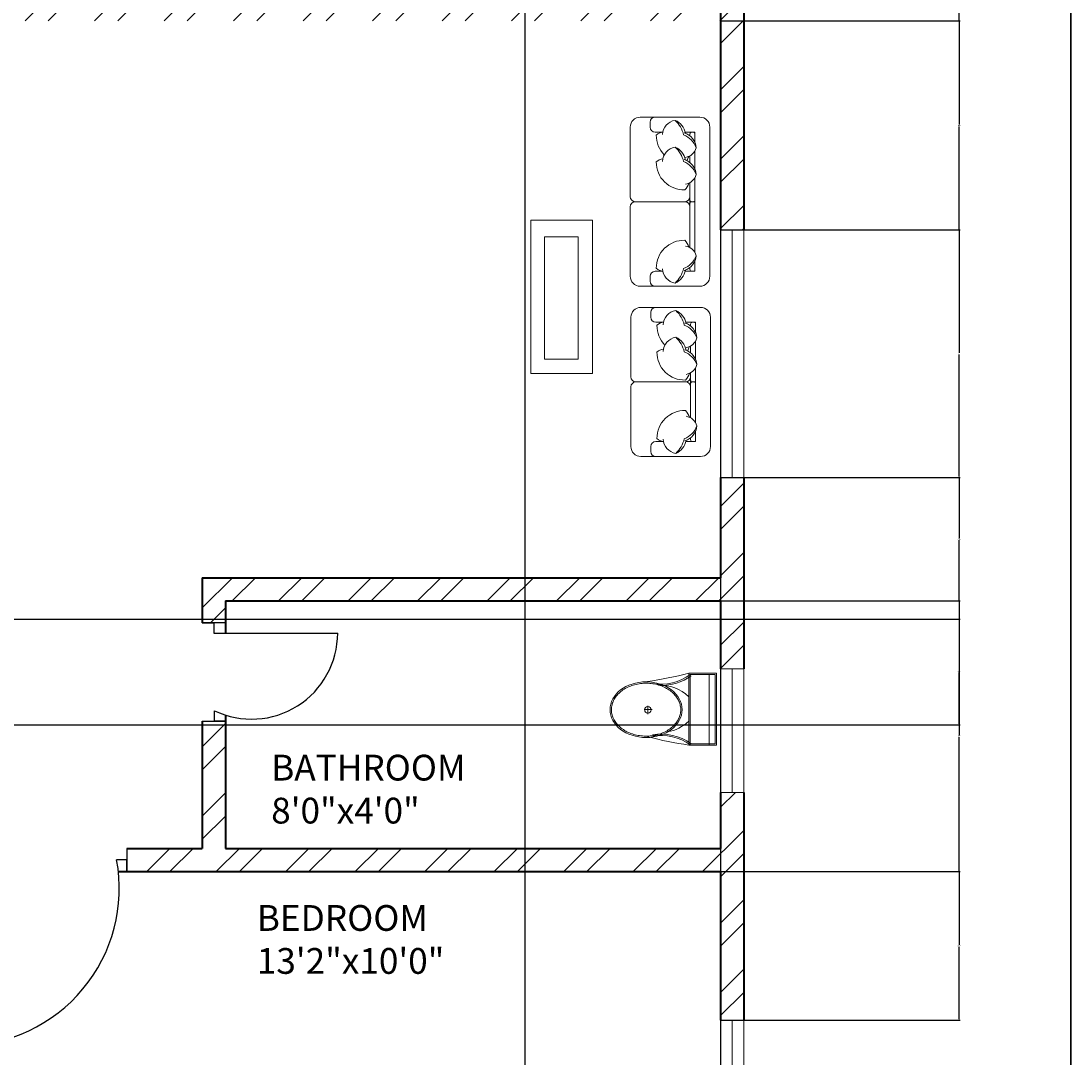
# Model space of a CAD drawing. Units: inches. Extents: x 2063 to 2617, y 1299 to 2210.
# Tile 5 of 22: x 2414 to 2617, y 1526 to 1727. Entities that reach past the tile are written whole.
import ezdxf

# ---------------------------------------------------------------- set-up
doc = ezdxf.new("R2010")
doc.units = ezdxf.units.IN
for name, color, linetype, lineweight in [('A-ANNO-DIMS', 2, 'Continuous', 18), ('A-ANNO-TTLB', 7, 'Continuous', 35), ('A-AREA-IDEN', 7, 'Continuous', 18), ('A-DOOR', 11, 'Continuous', 25), ('A-FLOR-FIXT', 8, 'Continuous', 18), ('A-FURN', 8, 'Continuous', 18), ('A-GLAZ', 123, 'Continuous', 18), ('A-WALL', 7, 'Continuous', 40)]:
    doc.layers.add(name, color=color, linetype=linetype, lineweight=lineweight)
doc.layers.add('A-WALL-PATT', color=215, linetype='Continuous', lineweight=13, true_color=0xa953a0)
doc.styles.get("Standard").update_dxf_attribs({"font": 'arial.ttf'})
doc.dimstyles.get("Standard").update_dxf_attribs({"dimtxt": 0.18, "dimasz": 0.18, "dimexe": 0.18, "dimexo": 0.0625, "dimgap": 0.09, "dimtad": 0, "dimtih": 1, "dimtoh": 1, "dimdec": 4, "dimzin": 0, "dimdsep": 46, "dimtxsty": 'Standard', "dimcen": 0.09, "dimadec": 0, "dimazin": 0, "dimtfac": 1, "dimtdec": 4, "dimtofl": 0, "dimtmove": 0, "dimatfit": 3, "dimfxl": 1, "dimtolj": 1, "dimtzin": 0, "dimarcsym": 0})

# ---------------------------------------------------------------- blocks, each defined once
blk = doc.blocks.new('A$C31115884')
for p, q in [((283.1, 497.7), (223.4, 497.7)), ((257.5, 466.4), (257.5, 523.2)), ((0, 200), (0, 0)), ((520, 200), (0, 200)), ((10, 190), (10, 10)), ((510, 190), (10, 190)), ((510, 10), (510, 190)), ((520, 0), (520, 200)), ((510, 54.5), (0, 54.5)), ((10, 10), (510, 10)), ((0, 0), (520, 0))]:
    blk.add_line(p, q)
blk.add_circle((255.6, 496.4), 23.6)
for centre, radius, start, end in [((2777.7, -204.6), 2807, 165.4549, 171.71327), ((-294.5, 403.3), 364.7, 324.20913, 9.34987), ((-294.5, 403.3), 374.7, 324.20913, 9.34987), ((805.8, 403.3), 364.7, 170.65013, 215.79087), ((3237, 905), 2807, 188.28673, 194.5451), ((139.5, 406.2), 293.5, 315.84364, 2.65635), ((805.8, 403.3), 374.7, 179.20365, 215.79087), ((383.6, 406.2), 293.5, 190.27735, 224.15636)]:
    blk.add_arc(centre, radius, start, end)
blk.add_ellipse((256.2, 509.9), major_axis=(0, -260.7), ratio=0.772727)
blk.add_open_spline([(256.2, 259.2), (263.1, 259.2), (270, 259.7), (287.8, 262.3), (298.7, 265.1), (319.9, 273.1), (330.2, 278.4), (350.1, 291.1), (359.7, 298.7), (377.7, 315.9), (386.2, 325.5), (401.7, 346.6), (408.8, 358.1), (421.3, 382.5), (426.8, 395.5), (435.9, 422.4), (439.5, 436.4), (444.8, 465.1), (446.5, 479.7), (447.9, 509.2), (447.6, 524), (445, 553.3), (442.7, 567.8), (436.3, 596), (432.1, 609.7), (421.9, 636), (416, 648.6), (402.5, 672.1), (395, 683), (378.6, 703), (369.8, 712.1), (351.1, 728), (341.3, 734.8), (320.9, 746.2), (310.4, 750.7), (288.9, 757.3), (278, 759.4), (256, 761), (245, 760.6), (223.1, 757.2), (212.3, 754.3), (191.1, 746.1), (180.8, 740.7), (160.9, 727.8), (151.4, 720.1), (133.5, 702.7), (125.1, 693), (109.6, 671.7), (102.6, 660.2), (90.2, 635.7), (84.9, 622.7), (76, 595.6), (72.4, 581.6), (67.2, 552.9), (65.6, 538.2), (64.4, 508.8), (64.8, 494), (67.5, 464.7), (69.9, 450.2), (76.6, 422), (80.8, 408.3), (91.1, 382.2), (97.2, 369.7), (110.8, 346.3), (118.4, 335.4), (134.8, 315.6), (143.7, 306.7), (162.4, 290.9), (172.3, 284.2), (192.8, 273), (203.3, 268.6), (224.8, 262.2), (235.8, 260.2), (249.9, 259.3), (253, 259.2), (256.2, 259.2)], degree=3, knots=[0, 0, 0, 0, 0.110105, 0.110105, 0.285049, 0.285049, 0.459994, 0.459994, 0.634938, 0.634938, 0.809882, 0.809882, 0.984827, 0.984827, 1.159771, 1.159771, 1.334715, 1.334715, 1.50966, 1.50966, 1.684604, 1.684604, 1.859549, 1.859549, 2.034493, 2.034493, 2.209437, 2.209437, 2.384382, 2.384382, 2.559326, 2.559326, 2.73427, 2.73427, 2.909215, 2.909215, 3.084159, 3.084159, 3.259103, 3.259103, 3.434048, 3.434048, 3.608992, 3.608992, 3.783936, 3.783936, 3.958881, 3.958881, 4.133825, 4.133825, 4.30877, 4.30877, 4.483714, 4.483714, 4.658658, 4.658658, 4.833603, 4.833603, 5.008547, 5.008547, 5.183491, 5.183491, 5.358436, 5.358436, 5.53338, 5.53338, 5.708324, 5.708324, 5.883269, 5.883269, 6.058213, 6.058213, 6.233158, 6.233158, 6.283185, 6.283185, 6.283185, 6.283185])
blk = doc.blocks.new('WIN-24IN')
for p, q in [((0, 24), (4.5, 24)), ((0, 24), (0, 0)), ((4.5, 24), (2.25, 24)), ((2.25, 24), (2.25, 0)), ((4.5, 24), (4.5, 0)), ((2.25, 0), (0, 0)), ((0, 0), (4.5, 0))]:
    blk.add_line(p, q)
blk = doc.blocks.new('TABLE-COFFEE')
for points in [[(0, 29.74), (11.98, 29.74), (11.98, 0), (0, 0)], [(2.66, 26.46), (2.66, 26.46), (2.66, 26.46), (2.66, 26.46)], [(2.66, 26.46), (2.66, 26.46), (2.66, 26.46), (2.66, 26.46)], [(2.66, 26.46), (2.66, 26.46), (2.66, 26.46), (2.66, 26.46)], [(2.66, 26.46), (9.18, 26.46), (9.18, 2.77), (2.66, 2.77)]]:
    blk.add_lwpolyline(points, close=True)
blk = doc.blocks.new('*D38')
at = {"layer": 'A-ANNO-DIMS', "color": 0, "lineweight": -2, "transparency": 16777216}
for p, q in [((2549.21, 1562.31), (2595.57, 1562.31)), ((2595.39, 1562.13), (2595.39, 1548.08)), ((2595.39, 1533.66), (2595.39, 1547.71)), ((2549.21, 1533.48), (2595.57, 1533.48))]:
    blk.add_line(p, q, dxfattribs=at)
at = {"layer": 'A-ANNO-DIMS', "color": 0, "transparency": 16777216}
for points in [[(2595.36, 1562.13), (2595.42, 1562.13), (2595.39, 1562.31)], [(2595.36, 1533.66), (2595.42, 1533.66), (2595.39, 1533.48)]]:
    blk.add_solid(points, dxfattribs=at)
at = {"layer": 'Defpoints', "color": 0, "transparency": 16777216}
for p in [(2549.14, 1562.31), (2595.39, 1562.31), (2549.14, 1533.48)]:
    blk.add_point(p, dxfattribs=at)
at = {"layer": 'A-ANNO-DIMS', "color": 0, "transparency": 16777216, "insert": (2595.39, 1547.9), "char_height": 0.18, "attachment_point": 5}
blk.add_mtext('\\A1;28.83', dxfattribs=at)
blk = doc.blocks.new('*D39')
at = {"layer": 'A-ANNO-DIMS', "color": 0, "lineweight": -2, "transparency": 16777216}
for p, q in [((2549.21, 1614.81), (2595.57, 1614.81)), ((2595.39, 1614.63), (2595.39, 1588.74)), ((2595.39, 1562.49), (2595.39, 1588.38)), ((2549.21, 1562.31), (2595.57, 1562.31))]:
    blk.add_line(p, q, dxfattribs=at)
at = {"layer": 'A-ANNO-DIMS', "color": 0, "transparency": 16777216}
for points in [[(2595.36, 1614.63), (2595.42, 1614.63), (2595.39, 1614.81)], [(2595.36, 1562.49), (2595.42, 1562.49), (2595.39, 1562.31)]]:
    blk.add_solid(points, dxfattribs=at)
at = {"layer": 'Defpoints', "color": 0, "transparency": 16777216}
for p in [(2549.14, 1614.81), (2595.39, 1614.81), (2549.14, 1562.31)]:
    blk.add_point(p, dxfattribs=at)
at = {"layer": 'A-ANNO-DIMS', "color": 0, "transparency": 16777216, "insert": (2595.39, 1588.56), "char_height": 0.18, "attachment_point": 5}
blk.add_mtext('\\A1;52.5', dxfattribs=at)
blk = doc.blocks.new('*D40')
at = {"layer": 'A-ANNO-DIMS', "color": 0, "lineweight": -2, "transparency": 16777216}
for p, q in [((2549.21, 1638.78), (2595.57, 1638.78)), ((2595.39, 1638.6), (2595.39, 1626.98)), ((2595.39, 1614.99), (2595.39, 1626.61)), ((2549.21, 1614.81), (2595.57, 1614.81))]:
    blk.add_line(p, q, dxfattribs=at)
at = {"layer": 'A-ANNO-DIMS', "color": 0, "transparency": 16777216}
for points in [[(2595.36, 1638.6), (2595.42, 1638.6), (2595.39, 1638.78)], [(2595.36, 1614.99), (2595.42, 1614.99), (2595.39, 1614.81)]]:
    blk.add_solid(points, dxfattribs=at)
at = {"layer": 'Defpoints', "color": 0, "transparency": 16777216}
for p in [(2549.14, 1638.78), (2595.39, 1638.78), (2549.14, 1614.81)]:
    blk.add_point(p, dxfattribs=at)
at = {"layer": 'A-ANNO-DIMS', "color": 0, "transparency": 16777216, "insert": (2595.39, 1626.79), "char_height": 0.18, "attachment_point": 5}
blk.add_mtext('\\A1;23.965', dxfattribs=at)
blk = doc.blocks.new('*D41')
at = {"layer": 'A-ANNO-DIMS', "color": 0, "lineweight": -2, "transparency": 16777216}
for p, q in [((2549.21, 1686.78), (2595.57, 1686.78)), ((2595.39, 1686.6), (2595.39, 1662.96)), ((2595.39, 1638.96), (2595.39, 1662.59)), ((2549.21, 1638.78), (2595.57, 1638.78))]:
    blk.add_line(p, q, dxfattribs=at)
at = {"layer": 'A-ANNO-DIMS', "color": 0, "transparency": 16777216}
for points in [[(2595.36, 1686.6), (2595.42, 1686.6), (2595.39, 1686.78)], [(2595.36, 1638.96), (2595.42, 1638.96), (2595.39, 1638.78)]]:
    blk.add_solid(points, dxfattribs=at)
at = {"layer": 'Defpoints', "color": 0, "transparency": 16777216}
for p in [(2549.14, 1686.78), (2595.39, 1686.78), (2549.14, 1638.78)]:
    blk.add_point(p, dxfattribs=at)
at = {"layer": 'A-ANNO-DIMS', "color": 0, "transparency": 16777216, "insert": (2595.39, 1662.78), "char_height": 0.18, "attachment_point": 5}
blk.add_mtext('\\A1;48', dxfattribs=at)
blk = doc.blocks.new('*D42')
at = {"layer": 'A-ANNO-DIMS', "color": 0, "lineweight": -2, "transparency": 16777216}
for p, q in [((2549.21, 1727.31), (2595.57, 1727.31)), ((2595.39, 1727.13), (2595.39, 1707.23)), ((2595.39, 1686.96), (2595.39, 1706.86)), ((2549.21, 1686.78), (2595.57, 1686.78))]:
    blk.add_line(p, q, dxfattribs=at)
at = {"layer": 'A-ANNO-DIMS', "color": 0, "transparency": 16777216}
for points in [[(2595.36, 1727.13), (2595.42, 1727.13), (2595.39, 1727.31)], [(2595.36, 1686.96), (2595.42, 1686.96), (2595.39, 1686.78)]]:
    blk.add_solid(points, dxfattribs=at)
at = {"layer": 'Defpoints', "color": 0, "transparency": 16777216}
for p in [(2549.14, 1727.31), (2595.39, 1727.31), (2549.14, 1686.78)]:
    blk.add_point(p, dxfattribs=at)
at = {"layer": 'A-ANNO-DIMS', "color": 0, "transparency": 16777216, "insert": (2595.39, 1707.04), "char_height": 0.18, "attachment_point": 5}
blk.add_mtext('\\A1;40.535', dxfattribs=at)
blk = doc.blocks.new('*D43')
at = {"layer": 'A-ANNO-DIMS', "color": 0, "lineweight": -2, "transparency": 16777216}
for p, q in [((2549.21, 1766.03), (2595.57, 1766.03)), ((2595.39, 1765.85), (2595.39, 1746.85)), ((2595.39, 1727.49), (2595.39, 1746.49)), ((2549.21, 1727.31), (2595.57, 1727.31))]:
    blk.add_line(p, q, dxfattribs=at)
at = {"layer": 'A-ANNO-DIMS', "color": 0, "transparency": 16777216}
for points in [[(2595.36, 1765.85), (2595.42, 1765.85), (2595.39, 1766.03)], [(2595.36, 1727.49), (2595.42, 1727.49), (2595.39, 1727.31)]]:
    blk.add_solid(points, dxfattribs=at)
at = {"layer": 'Defpoints', "color": 0, "transparency": 16777216}
for p in [(2549.14, 1766.03), (2595.39, 1766.03), (2549.14, 1727.31)]:
    blk.add_point(p, dxfattribs=at)
at = {"layer": 'A-ANNO-DIMS', "color": 0, "transparency": 16777216, "insert": (2595.39, 1746.67), "char_height": 0.18, "attachment_point": 5}
blk.add_mtext('\\A1;38.72', dxfattribs=at)
blk = doc.blocks.new('*D52')
at = {"layer": 'A-ANNO-DIMS', "color": 0, "lineweight": -2, "transparency": 16777216}
for p, q in [((2511.17, 2124.25), (2511.17, 1317.7)), ((2549.14, 2124.25), (2549.14, 1317.7)), ((2511.35, 1317.88), (2529.69, 1317.88)), ((2548.96, 1317.88), (2530.62, 1317.88))]:
    blk.add_line(p, q, dxfattribs=at)
at = {"layer": 'A-ANNO-DIMS', "color": 0, "transparency": 16777216}
for points in [[(2511.35, 1317.91), (2511.35, 1317.85), (2511.17, 1317.88)], [(2548.96, 1317.91), (2548.96, 1317.85), (2549.14, 1317.88)]]:
    blk.add_solid(points, dxfattribs=at)
at = {"layer": 'Defpoints', "color": 0, "transparency": 16777216}
for p in [(2511.17, 2124.31), (2549.14, 2124.31), (2549.14, 1317.88)]:
    blk.add_point(p, dxfattribs=at)
at = {"layer": 'A-ANNO-DIMS', "color": 0, "transparency": 16777216, "insert": (2530.16, 1317.88), "char_height": 0.18, "attachment_point": 5}
blk.add_mtext('\\A1;37.974', dxfattribs=at)
blk = doc.blocks.new('*D68')
at = {"layer": 'A-ANNO-DIMS', "color": 0, "lineweight": -2, "transparency": 16777216}
for p, q in [((2228.21, 1611.27), (2595.57, 1611.27)), ((2595.39, 1611.09), (2595.39, 1601.22)), ((2595.39, 1590.99), (2595.39, 1600.86)), ((2228.21, 1590.81), (2595.57, 1590.81))]:
    blk.add_line(p, q, dxfattribs=at)
at = {"layer": 'A-ANNO-DIMS', "color": 0, "transparency": 16777216}
for points in [[(2595.36, 1611.09), (2595.42, 1611.09), (2595.39, 1611.27)], [(2595.36, 1590.99), (2595.42, 1590.99), (2595.39, 1590.81)]]:
    blk.add_solid(points, dxfattribs=at)
at = {"layer": 'Defpoints', "color": 0, "transparency": 16777216}
for p in [(2228.14, 1611.27), (2595.39, 1611.27), (2228.14, 1590.81)]:
    blk.add_point(p, dxfattribs=at)
at = {"layer": 'A-ANNO-DIMS', "color": 0, "transparency": 16777216, "insert": (2595.39, 1601.04), "char_height": 0.18, "attachment_point": 5}
blk.add_mtext('\\A1;20.46', dxfattribs=at)

msp = doc.modelspace()

# ---------------------------------------------------------------- hatches: boundary and pattern name
at = {"layer": 'A-WALL-PATT'}
h = msp.add_hatch(dxfattribs=at)
h.set_pattern_fill('ANSI32', color=256)
h.paths.add_polyline_path([(2553.6442, 2128.8122), (2511.1703, 2128.8122), (2511.1703, 2124.3122), (2549.1442, 2124.3122), (2549.1442, 2095.662), (2553.6442, 2095.662)])
h.paths.add_polyline_path([(2553.6442, 2035.662), (2549.1442, 2035.662), (2549.1442, 1980.3122), (2503.7214, 1980.3122), (2503.7214, 1975.8122), (2549.1442, 1975.8122), (2549.1442, 1962.9693), (2553.6442, 1962.9693)])
h.paths.add_polyline_path([(2553.6442, 1938.9693), (2549.1442, 1938.9693), (2549.1442, 1927.8122), (2477.1442, 1927.8122), (2477.1442, 1975.8122), (2481.2918, 1975.8122), (2481.2918, 1980.3122), (2453.2648, 1980.3122), (2453.2648, 1975.8122), (2472.6442, 1975.8122), (2472.6442, 1868.3122), (2400.6442, 1868.3122), (2400.6442, 1861.3782), (2405.1442, 1861.3782), (2405.1442, 1863.8122), (2480.9699, 1863.8122), (2480.9699, 1866.0622), (2480.9699, 1868.3122), (2477.1442, 1868.3122), (2477.1442, 1923.3122), (2549.1442, 1923.3122), (2549.1442, 1908.8504), (2553.6442, 1908.8504)])
h.paths.add_polyline_path([(2553.6442, 1884.8504), (2549.1442, 1884.8504), (2549.1442, 1868.3122), (2501.0636, 1868.3122), (2501.0636, 1863.8122), (2549.1442, 1863.8122), (2549.1442, 1826.0298), (2553.6442, 1826.0298)])
h.paths.add_polyline_path([(2388.1504, 1980.3122), (2340.6442, 1980.3122), (2340.6442, 2124.3122), (2358.7501, 2124.3122), (2358.7501, 2128.8122), (2316.3482, 2128.8122), (2316.3482, 2124.3122), (2336.1442, 2124.3122), (2336.1442, 1980.3122), (2289.1737, 1980.3122), (2289.1737, 1975.8122), (2336.1442, 1975.8122), (2336.1442, 1619.3122), (2333.1433, 1619.3122), (2333.1433, 1614.8122), (2344.1671, 1614.8122), (2344.1671, 1617.0622), (2344.1671, 1619.3122), (2340.6442, 1619.3122), (2340.6442, 1975.8122), (2388.1504, 1975.8122), (2388.1504, 1978.0622)])
h.paths.add_polyline_path([(2290.1442, 1614.8122), (2301.4594, 1614.8122), (2301.4594, 1617.0622), (2301.4594, 1619.3122), (2285.6442, 1619.3122), (2285.6442, 1566.8122), (2280.8619, 1566.8122), (2280.8619, 1564.5622), (2280.8619, 1562.3122), (2285.6442, 1562.3122), (2285.6442, 1442.3122), (2281.7879, 1442.3122), (2281.7879, 1437.8122), (2285.6442, 1437.8122), (2285.6442, 1401.8122), (2290.1442, 1401.8122)])
h.paths.add_polyline_path([(2549.1442, 1731.8122), (2405.1442, 1731.8122), (2405.1442, 1834.4638), (2402.8942, 1834.4638), (2400.6442, 1834.4638), (2400.6442, 1727.3122), (2549.1442, 1727.3122)])
h.paths.add_polyline_path([(2553.6442, 1766.0298), (2551.3942, 1766.0298), (2549.1442, 1766.0298), (2549.1442, 1686.7767), (2553.6442, 1686.7767)])
h.paths.add_polyline_path([(2553.6442, 1638.7767), (2551.3942, 1638.7767), (2549.1442, 1638.7767), (2549.1442, 1619.3122), (2448.6442, 1619.3122), (2448.6442, 1610.5671), (2450.8942, 1610.5671), (2453.1442, 1610.5671), (2453.1442, 1614.8122), (2549.1442, 1614.8122), (2549.1442, 1601.6421), (2553.6442, 1601.6421)])
h.paths.add_polyline_path([(2553.6442, 1577.6421), (2551.3942, 1577.6421), (2549.1442, 1577.6421), (2549.1442, 1566.8122), (2453.1442, 1566.8122), (2453.1442, 1591.5045), (2451.0335, 1591.5045), (2448.6442, 1591.5045), (2448.6442, 1566.8122), (2434.0475, 1566.8122), (2434.0475, 1562.3122), (2549.1442, 1562.3122), (2549.1442, 1533.48), (2553.6442, 1533.48)])
h.paths.add_polyline_path([(2553.6442, 1473.48), (2549.1442, 1473.48), (2549.1442, 1442.3122), (2502.6258, 1442.3122), (2502.6258, 1437.8122), (2549.1442, 1437.8122), (2549.1442, 1401.8122), (2553.6442, 1401.8122)])
h.paths.add_polyline_path([(2395.6442, 1562.3122), (2400.0901, 1562.3122), (2400.0901, 1564.5622), (2400.0901, 1566.8122), (2395.6442, 1566.8122), (2395.6442, 1619.3122), (2379.1127, 1619.3122), (2379.1127, 1614.8122), (2391.1442, 1614.8122), (2391.1442, 1401.8122), (2395.6442, 1401.8122), (2395.6442, 1437.8122), (2399.2425, 1437.8122), (2399.2425, 1440.0622), (2399.2425, 1442.3122), (2395.6442, 1442.3122)])
h.paths.add_polyline_path([(2442.6258, 1442.3122), (2419.6262, 1442.3122), (2419.6262, 1437.8122), (2442.6258, 1437.8122), (2442.6258, 1440.0622)])
h.paths.add_polyline_path([(2127.6442, 1480.2532), (2125.3942, 1480.2532), (2123.1442, 1480.2532), (2123.1442, 1401.8122), (2127.6442, 1401.8122), (2127.6442, 1437.8122), (2145.1538, 1437.8122), (2145.1538, 1440.0622), (2145.1538, 1442.3122), (2127.6442, 1442.3122)])
h.paths.add_polyline_path([(2259.809, 1442.3122), (2205.1538, 1442.3122), (2205.1538, 1437.8122), (2259.809, 1437.8122), (2259.809, 1440.0622)])
h.paths.add_polyline_path([(2127.6442, 1659.7652), (2123.1442, 1659.7652), (2123.1442, 1605.5161), (2125.3942, 1605.5161), (2127.6442, 1605.5161), (2127.6442, 1614.8122), (2223.6442, 1614.8122), (2223.6442, 1611.2723), (2228.1442, 1611.2723), (2228.1442, 1619.3122), (2127.6442, 1619.3122)])
h.paths.add_polyline_path([(2244.8673, 1566.8122), (2228.1442, 1566.8122), (2228.1442, 1590.8122), (2225.8942, 1590.8122), (2223.6442, 1590.8122), (2223.6442, 1566.8122), (2127.6442, 1566.8122), (2127.6442, 1581.5161), (2123.1442, 1581.5161), (2123.1442, 1540.2532), (2127.6442, 1540.2532), (2127.6442, 1562.3122), (2244.8673, 1562.3122), (2244.8673, 1564.5622)])
h.paths.add_polyline_path([(2172.5174, 1868.3122), (2127.6442, 1868.3122), (2127.6442, 1886.5833), (2123.1442, 1886.5833), (2123.1442, 1832.6633), (2127.6442, 1832.6633), (2127.6442, 1863.8122), (2172.5174, 1863.8122), (2172.5174, 1866.0622)])
h.paths.add_polyline_path([(2276.1442, 1868.3122), (2204.1442, 1868.3122), (2204.1442, 1923.3122), (2204.1442, 1975.8122), (2224.8362, 1975.8122), (2224.8362, 1978.1097), (2224.8362, 1980.3122), (2195.0729, 1980.3122), (2195.0729, 1978.0622), (2195.0729, 1975.8122), (2199.6442, 1975.8122), (2199.6442, 1927.8122), (2127.6442, 1927.8122), (2127.6442, 1942.3492), (2123.1442, 1942.3492), (2123.1442, 1910.5833), (2127.6442, 1910.5833), (2127.6442, 1923.3122), (2199.6442, 1923.3122), (2199.6442, 1868.3122), (2194.8228, 1868.3122), (2194.8228, 1864.7337), (2194.8228, 1863.8122), (2271.6442, 1863.8122), (2271.6442, 1860.0507), (2276.1442, 1860.0507)])
h.paths.add_polyline_path([(2276.1442, 1829.994), (2273.8942, 1829.994), (2271.6442, 1829.994), (2271.6442, 1731.8122), (2127.6442, 1731.8122), (2127.6442, 1772.6633), (2123.1442, 1772.6633), (2123.1442, 1707.7652), (2127.6442, 1707.7652), (2127.6442, 1727.3122), (2276.1442, 1727.3122)])
h.paths.add_polyline_path([(2127.6442, 2022.1152), (2123.1442, 2022.1152), (2123.1442, 1966.3492), (2127.6442, 1966.3492), (2127.6442, 1975.8122), (2174.2082, 1975.8122), (2174.2082, 1978.0622), (2174.2082, 1980.3122), (2127.6442, 1980.3122)])
h.paths.add_polyline_path([(2361.9755, 1678.588), (2398.4558, 1678.588), (2398.4558, 1697.2453), (2361.9755, 1697.2453)], flags=9)
h.paths.add_polyline_path([(2351.5397, 1780.4072), (2386.1987, 1780.4072), (2386.1987, 1790.7107), (2351.5397, 1790.7107)], flags=25)
h.paths.add_polyline_path([(2350.6753, 1940.9321), (2387.6024, 1940.9321), (2387.6024, 1959.5894), (2350.6753, 1959.5894)], flags=25)
h.paths.add_polyline_path([(2254.9545, 1684.638), (2295.0943, 1684.638), (2295.0943, 1703.2953), (2254.9545, 1703.2953)], flags=9)
h.paths.add_polyline_path([(2282.4946, 1782.4438), (2317.1535, 1782.4438), (2317.1535, 1792.7474), (2282.4946, 1792.7474)], flags=9)
h.paths.add_polyline_path([(2270.327, 1939.2854), (2307.254, 1939.2854), (2307.254, 1957.9428), (2270.327, 1957.9428)], flags=9)

# ---------------------------------------------------------------- linework, layer by layer
at = {"layer": 'A-ANNO-TTLB'}
msp.add_lwpolyline([(2062.5792, 2209.6485), (2617.0648, 2209.6485), (2617.0648, 1299.1125), (2062.5792, 1299.1125)], close=True, dxfattribs=at)
at = {"layer": 'A-DOOR'}
for p, q in [((2453.1442, 1610.5671), (2448.6442, 1610.5671)), ((2448.6442, 1610.5671), (2450.8942, 1610.5671)), ((2450.8942, 1610.5671), (2450.8942, 1608.5671)), ((2450.8942, 1608.5671), (2474.8942, 1608.5671)), ((2451.0335, 1591.5045), (2451.0335, 1593.5045)), ((2448.6442, 1591.5045), (2453.1442, 1591.5045)), ((2453.1442, 1591.5045), (2451.0335, 1591.5045)), ((2434.0475, 1566.8122), (2434.0475, 1562.3122)), ((2434.0475, 1564.5622), (2432.0475, 1564.5622)), ((2434.0475, 1562.3122), (2434.0475, 1564.5622))]:
    msp.add_line(p, q, dxfattribs=at)
for centre, radius, start, end in [((2458.2096, 1608.5671), 16.6847, 244.526088, 0), ((2402.0901, 1559.0267), 30.4645, 270, 10.468944)]:
    msp.add_arc(centre, radius, start, end, dxfattribs=at)
at = {"layer": 'A-FURN', "ltscale": 0.03}
for points in [[(2531.6192, 1691.2936, -0.41421356), (2532.5836, 1692.258, -0.41421356), (2531.6192, 1693.2224), (2531.6192, 1706.7244, -0.41421356), (2533.5481, 1708.6532), (2545.1212, 1708.6532, -0.41421356), (2547.05, 1706.7244), (2547.05, 1677.7916, -0.41421356), (2545.1212, 1675.8628), (2533.5481, 1675.8628, -0.41421356), (2531.6192, 1677.7916), (2531.6192, 1691.2936, -0.41421356), (2532.5836, 1692.258, -0.41421356), (2531.6192, 1693.2224)], [(2531.7488, 1656.3327, -0.41421356), (2532.7132, 1657.2972, -0.41421356), (2531.7488, 1658.2616), (2531.7488, 1669.8347, -0.41421356), (2533.6776, 1671.7635), (2545.2507, 1671.7635, -0.41421356), (2547.1796, 1669.8347), (2547.1796, 1644.7596, -0.41421356), (2545.2507, 1642.8308), (2533.6776, 1642.8308, -0.41421356), (2531.7488, 1644.7596), (2531.7488, 1656.3327, -0.41421356), (2532.7132, 1657.2972, -0.41421356), (2531.7488, 1658.2616)]]:
    msp.add_lwpolyline(points, format="xyb", dxfattribs=at)
at = {"layer": 'A-FURN'}
for points in [[(2537.9356, 1705.7599), (2536.4413, 1705.7599, -0.41421356), (2535.4769, 1706.7244), (2535.4769, 1707.6888, -0.41421356), (2536.4413, 1708.6532)], [(2537.8772, 1705.2759, -0.35677236), (2540.3082, 1708.0394, -0.24954205), (2542.3115, 1705.5355, 9.61688035)], [(2540.3082, 1708.0394, -0.14772988), (2541.9656, 1705.2207, -0.21334276), (2544.3966, 1702.7336, -0.17866181)], [(2537.936, 1705.762, 0.16554063), (2536.6617, 1705.1654, 0.20023115), (2538.2137, 1701.337, 0.12152332)], [(2542.0977, 1705.6101, -0.30666349), (2544.3966, 1702.7336, -0.30632997), (2542.2971, 1700.8544, 0.87284716)], [(2544.1567, 1703.7311), (2544.1567, 1705.7599), (2542.2614, 1705.7599, -0.41421356)], [(2543.1923, 1705.024), (2543.1923, 1705.3742, -0.41421356), (2543.5781, 1705.7599), (2543.771, 1705.7599, -0.41421356), (2544.1567, 1705.3742)], [(2544.1567, 1705.3742), (2544.1567, 1703.7311, -0.41421356)], [(2537.8772, 1700.0806, -0.35677236), (2540.3082, 1702.8441, -0.24954205), (2542.3115, 1700.3401, 9.61688035)], [(2540.3082, 1702.8441, -0.14772988), (2541.9656, 1700.0254, -0.21334276), (2544.3966, 1697.5382, -0.17866181)], [(2544.1567, 1702.1266), (2544.1567, 1698.5357, -0.41421356)], [(2537.936, 1700.5667, 0.16554063), (2536.6617, 1699.9701, 0.42598917), (2542.1866, 1694.5537, 0.12152332), (2542.9481, 1695.8395, -7.11546429)], [(2542.0977, 1700.4148, -0.30666349), (2544.3966, 1697.5382, -0.30632997), (2542.2971, 1695.6591, 0.87284716)], [(2542.5711, 1700.2262, 0.07186538), (2542.9481, 1701.0348, -7.11546429)], [(2543.1923, 1699.8287), (2543.1923, 1701.1555, -0.41421356)], [(2544.1567, 1696.9313), (2544.1567, 1692.6438, -0.41421356), (2543.771, 1692.258), (2543.5781, 1692.258, -0.41421356), (2543.1923, 1692.6438), (2543.1923, 1695.9602, -0.41421356)], [(2543.1923, 1693.2224, -0.41421356), (2542.2279, 1692.258), (2532.5836, 1692.258, -0.41421356)], [(2543.1923, 1691.2936, 0.41421356), (2542.2279, 1692.258), (2532.5836, 1692.258, 0.41421356)], [(2543.1923, 1693.2224, -0.41421356), (2542.2279, 1692.258)], [(2543.1923, 1691.2936, 0.41421356), (2542.2279, 1692.258)], [(2544.1567, 1682.3894), (2544.1567, 1691.8722, 0.41421356), (2543.771, 1692.258), (2543.5781, 1692.258, 0.41421356), (2543.1923, 1691.8722), (2543.1923, 1683.3605, 0.41421356)], [(2537.936, 1678.754, -0.16554063), (2536.6617, 1679.3506, -0.42598917), (2542.1866, 1684.767, -0.12152332), (2542.9481, 1683.4812, 7.11546429)], [(2542.0977, 1678.9059, 0.30666349), (2544.3966, 1681.7824, 0.30632997), (2542.2971, 1683.6616, -0.87284716)], [(2540.3082, 1676.4766, 0.14772988), (2541.9656, 1679.2953, 0.21334276), (2544.3966, 1681.7824, 0.17866181)], [(2543.1923, 1679.492), (2543.1923, 1679.1418, 0.41421356), (2543.5781, 1678.7561), (2543.771, 1678.7561, 0.41421356), (2544.1567, 1679.1418)], [(2544.1567, 1679.1418), (2544.1567, 1680.785, 0.41421356)], [(2536.4413, 1675.8628, -0.41421356), (2535.4769, 1676.8272), (2535.4769, 1677.7916, -0.41421356), (2536.4413, 1678.7561), (2537.9356, 1678.7561)], [(2537.8772, 1679.2401, 0.35677236), (2540.3082, 1676.4766, 0.24954205), (2542.3115, 1678.9805, -9.61688035)], [(2538.0652, 1668.8702), (2536.5709, 1668.8702, -0.41421356), (2535.6065, 1669.8347), (2535.6065, 1670.7991, -0.41421356), (2536.5709, 1671.7635)], [(2538.0068, 1668.3863, -0.35677236), (2540.4377, 1671.1497, -0.24954205), (2542.441, 1668.6458, 9.61688035)], [(2540.4377, 1671.1497, -0.14772988), (2542.0952, 1668.331, -0.21334276), (2544.5261, 1665.8439, -0.17866181)], [(2538.0656, 1668.8723, 0.16554063), (2536.7913, 1668.2757, 0.20023115), (2538.3433, 1664.4473, 0.12152332)], [(2542.2273, 1668.7204, -0.30666349), (2544.5261, 1665.8439, -0.30632997), (2542.4267, 1663.9647, 0.87284716)], [(2544.2863, 1666.8414), (2544.2863, 1668.8702), (2542.391, 1668.8702, -0.41421356)], [(2543.3219, 1668.1343), (2543.3219, 1668.4845, -0.41421356), (2543.7076, 1668.8702), (2543.9005, 1668.8702, -0.41421356), (2544.2863, 1668.4845)], [(2544.2863, 1668.4845), (2544.2863, 1666.8414, -0.41421356)], [(2538.0068, 1663.1909, -0.35677236), (2540.4377, 1665.9544, -0.24954205), (2542.441, 1663.4504, 9.61688035)], [(2540.4377, 1665.9544, -0.14772988), (2542.0952, 1663.1357, -0.21334276), (2544.5261, 1660.6486, -0.17866181)], [(2544.2863, 1665.2369), (2544.2863, 1661.646, -0.41421356)], [(2538.0656, 1663.677, 0.16554063), (2536.7913, 1663.0804, 0.42598917), (2542.3162, 1657.664, 0.12152332), (2543.0777, 1658.9498, -7.11546429)], [(2542.2273, 1663.5251, -0.30666349), (2544.5261, 1660.6486, -0.30632997), (2542.4267, 1658.7694, 0.87284716)], [(2542.7006, 1663.3365, 0.07186538), (2543.0777, 1664.1451, -7.11546429)], [(2543.3219, 1662.939), (2543.3219, 1664.2658, -0.41421356)], [(2544.2863, 1660.0416), (2544.2863, 1657.6829, -0.41421356), (2543.9005, 1657.2972), (2543.7076, 1657.2972, -0.41421356), (2543.3219, 1657.6829), (2543.3219, 1659.0705, -0.41421356)], [(2543.3219, 1658.2616, -0.41421356), (2542.3574, 1657.2972), (2532.7132, 1657.2972, -0.41421356)], [(2543.3219, 1656.3327, 0.41421356), (2542.3574, 1657.2972), (2532.7132, 1657.2972, 0.41421356)], [(2543.3219, 1658.2616, -0.41421356), (2542.3574, 1657.2972)], [(2543.3219, 1656.3327, 0.41421356), (2542.3574, 1657.2972)], [(2544.2863, 1649.3574), (2544.2863, 1656.9114, 0.41421356), (2543.9005, 1657.2972), (2543.7076, 1657.2972, 0.41421356), (2543.3219, 1656.9114), (2543.3219, 1650.3285, 0.41421356)], [(2538.0656, 1645.722, -0.16554063), (2536.7913, 1646.3186, -0.42598917), (2542.3162, 1651.735, -0.12152332), (2543.0777, 1650.4492, 7.11546429)], [(2542.2273, 1645.8739, 0.30666349), (2544.5261, 1648.7504, 0.30632997), (2542.4267, 1650.6296, -0.87284716)], [(2540.4377, 1643.4446, 0.14772988), (2542.0952, 1646.2633, 0.21334276), (2544.5261, 1648.7504, 0.17866181)], [(2544.2863, 1646.1098), (2544.2863, 1647.753, 0.41421356)], [(2536.5709, 1642.8308, -0.41421356), (2535.6065, 1643.7952), (2535.6065, 1644.7596, -0.41421356), (2536.5709, 1645.7241), (2538.0652, 1645.7241)], [(2538.0068, 1646.2081, 0.35677236), (2540.4377, 1643.4446, 0.24954205), (2542.441, 1645.9485, -9.61688035)], [(2543.3219, 1646.46), (2543.3219, 1646.1098, 0.41421356), (2543.7076, 1645.7241), (2543.9005, 1645.7241, 0.41421356), (2544.2863, 1646.1098)]]:
    msp.add_lwpolyline(points, format="xyb", dxfattribs=at)
for points in [[(2544.1567, 1698.5357), (2544.1567, 1702.1266)], [(2544.1567, 1682.3894), (2544.1567, 1696.9313)], [(2542.2614, 1678.7561), (2544.1567, 1678.7561), (2544.1567, 1680.785)], [(2544.2863, 1661.646), (2544.2863, 1665.2369)], [(2544.2863, 1649.3574), (2544.2863, 1660.0416)], [(2542.391, 1645.7241), (2544.2863, 1645.7241), (2544.2863, 1647.753)]]:
    msp.add_lwpolyline(points, dxfattribs=at)
for points in [[(2544.1567, 1691.8722), (2544.1567, 1692.6438, -0.41421356), (2543.771, 1692.258), (2543.5781, 1692.258, -0.41421356), (2543.1923, 1692.6438), (2543.1923, 1691.8722, -0.41421356), (2543.5781, 1692.258), (2543.771, 1692.258, -0.41421356)], [(2544.2863, 1656.9114), (2544.2863, 1657.6829, -0.41421356), (2543.9005, 1657.2972), (2543.7076, 1657.2972, -0.41421356), (2543.3219, 1657.6829), (2543.3219, 1656.9114, -0.41421356), (2543.7076, 1657.2972), (2543.9005, 1657.2972, -0.41421356)]]:
    msp.add_lwpolyline(points, format="xyb", close=True, dxfattribs=at)
at = {"layer": 'A-GLAZ'}
for p, q in [((2551.3942, 1686.7767), (2549.1442, 1686.7767)), ((2549.1442, 1686.7767), (2553.6442, 1686.7767)), ((2549.1442, 1686.7767), (2549.1442, 1640.6277)), ((2551.3942, 1638.7767), (2551.3942, 1686.7767)), ((2553.6442, 1686.7767), (2553.6442, 1638.7767)), ((2549.1442, 1640.6277), (2549.1442, 1638.7767)), ((2549.1442, 1638.7767), (2553.6442, 1638.7767)), ((2553.6442, 1638.7767), (2551.3942, 1638.7767)), ((2549.1442, 1533.48), (2553.6442, 1533.48)), ((2549.1442, 1533.48), (2549.1442, 1473.48)), ((2553.6442, 1533.48), (2551.3942, 1533.48)), ((2551.3942, 1533.48), (2551.3942, 1473.48)), ((2553.6442, 1533.48), (2553.6442, 1473.48))]:
    msp.add_line(p, q, dxfattribs=at)
at = {"layer": 'A-WALL'}
for p, q in [((2549.1442, 1766.0298), (2549.1442, 1686.7767)), ((2553.6442, 1766.0298), (2553.6442, 1686.7767)), ((2549.1442, 1638.7767), (2549.1442, 1619.3122)), ((2553.6442, 1638.7767), (2553.6442, 1601.6421)), ((2448.6442, 1619.3122), (2549.1442, 1619.3122)), ((2448.6442, 1619.3122), (2448.6442, 1610.5671)), ((2453.1442, 1614.8122), (2549.1442, 1614.8122)), ((2453.1442, 1614.8122), (2453.1442, 1608.5671)), ((2549.1442, 1614.8122), (2549.1442, 1601.6421)), ((2453.1442, 1592.67), (2453.1442, 1566.8122)), ((2448.6442, 1591.5045), (2448.6442, 1566.8122)), ((2549.1442, 1577.6421), (2549.1442, 1566.8122)), ((2553.6442, 1577.6421), (2553.6442, 1533.48)), ((2434.0475, 1566.8122), (2448.6442, 1566.8122)), ((2453.1442, 1566.8122), (2549.1442, 1566.8122)), ((2432.377, 1562.3122), (2549.1442, 1562.3122)), ((2549.1442, 1562.3122), (2549.1442, 1533.48))]:
    msp.add_line(p, q, dxfattribs=at)

# ---------------------------------------------------------------- block references
at = {"layer": 'A-FLOR-FIXT', "xscale": 0.0268011493576733, "yscale": 0.0268011493576733, "zscale": 0.0268011493576733, "rotation": 89.99999999999999}
msp.add_blockref('A$C31115884', (2548.3487, 1586.8556), dxfattribs=at)
at = {"layer": 'A-FURN'}
msp.add_blockref('TABLE-COFFEE', (2512.333, 1658.952), dxfattribs=at)
at = {"layer": 'A-GLAZ', "extrusion": (0, 0, -1), "zscale": -1, "rotation": 180}
msp.add_blockref('WIN-24IN', (-2549.144, 1601.6424), dxfattribs=at)

# ---------------------------------------------------------------- texts
at = {"layer": 'A-AREA-IDEN', "char_height": 5, "attachment_point": 1}
for s, width, insert in [('BATHROOM\\P8\'0"x4\'0"', 186.413694, (2462.0059, 1584.9748)), ('BEDROOM\\P13\'2"x10\'0"', 249.482519, (2459.2126, 1555.8151))]:
    msp.add_mtext_dynamic_manual_height_columns(s, width=width, gutter_width=12.5, heights=[0], dxfattribs=dict(at, insert=insert))

# ---------------------------------------------------------------- dimensions: what is measured, and where the dimension line sits
at = {"layer": 'A-ANNO-DIMS'}
dim = msp.add_linear_dim(base=(2549.1442, 1317.8821), p1=(2511.1703, 2124.3122), p2=(2549.1442, 2124.3122), dimstyle='Standard', override={"dimdec": 3, "dimlfac": 1, "dimrnd": 0, "dimzin": 0, "dimdsep": 46, "dimlunit": 2}, dxfattribs=at)
dim.commit()
dim.dimension.update_dxf_attribs({"geometry": '*D52', "text_midpoint": (2530.1573, 1317.8821)})
for base, p1, p2, override, picture, middle in [((2595.3943, 1766.0298), (2549.1442, 1727.3122), (2549.1442, 1766.0298), {"dimdec": 2, "dimlfac": 1, "dimrnd": 0, "dimzin": 0, "dimdsep": 46, "dimlunit": 2}, '*D43', (2595.3943, 1746.671)), ((2595.39425, 1727.31218), (2549.14425, 1686.77674), (2549.14425, 1727.31218), {"dimdec": 3, "dimlfac": 1, "dimrnd": 0, "dimzin": 0, "dimdsep": 46, "dimlunit": 2}, '*D42', (2595.39425, 1707.04446)), ((2595.3943, 1686.7767), (2549.1442, 1638.7767), (2549.1442, 1686.7767), {"dimdec": 0, "dimlfac": 1, "dimrnd": 0, "dimzin": 0, "dimdsep": 46, "dimlunit": 2}, '*D41', (2595.3943, 1662.7767)), ((2595.39425, 1638.77674), (2549.14425, 1614.81218), (2549.14425, 1638.77674), {"dimdec": 3, "dimlfac": 1, "dimrnd": 0, "dimzin": 0, "dimdsep": 46, "dimlunit": 2}, '*D40', (2595.39425, 1626.79446)), ((2595.3943, 1614.8122), (2549.1442, 1562.3122), (2549.1442, 1614.8122), {"dimdec": 1, "dimlfac": 1, "dimrnd": 0, "dimzin": 0, "dimdsep": 46, "dimlunit": 2}, '*D39', (2595.3943, 1588.5622)), ((2595.3943, 1611.2723), (2228.1442, 1590.8122), (2228.1442, 1611.2723), {"dimdec": 2, "dimlfac": 1, "dimrnd": 0, "dimzin": 0, "dimdsep": 46, "dimlunit": 2}, '*D68', (2595.3943, 1601.0422)), ((2595.3943, 1562.3122), (2549.1442, 1533.48), (2549.1442, 1562.3122), {"dimdec": 2, "dimlfac": 1, "dimrnd": 0, "dimzin": 0, "dimdsep": 46, "dimlunit": 2}, '*D38', (2595.3943, 1547.8961))]:
    dim = msp.add_linear_dim(base=base, p1=p1, p2=p2, angle=90, dimstyle='Standard', override=override, dxfattribs=at)
    dim.commit()
    dim.dimension.update_dxf_attribs({"geometry": picture, "text_midpoint": middle})

doc.saveas('drawing.dxf')
